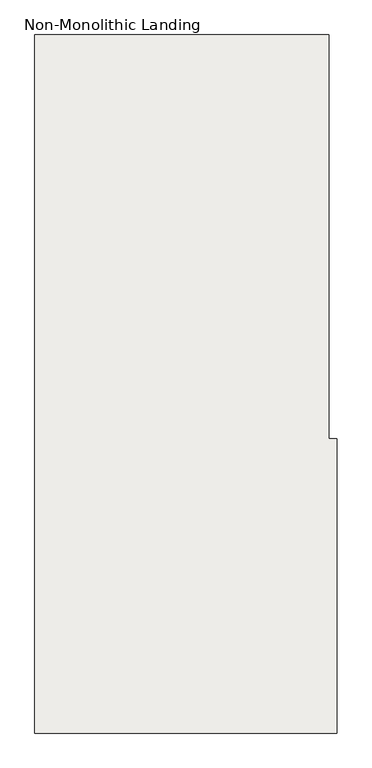
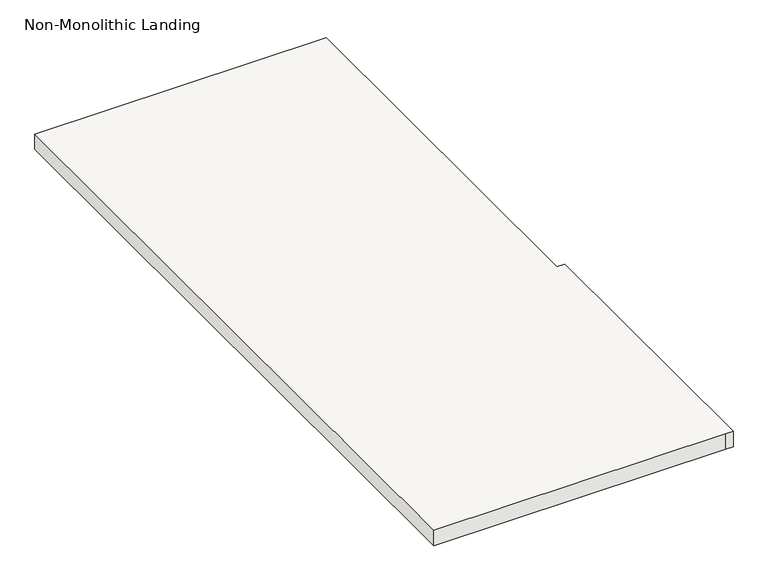
"""IFC4 building model written with IfcOpenShell, lengths in millimetres: slab geometry, Non-Monolithic Landing."""

from ifc_helpers import new_model, si_unit, origin, place, context, project, spatial, faceted_brep, source, transform, mapped, element, save


def non_monolithic_landing_bb243dde(model_context):
    return source(origin(), model_context, "Body", "Brep", [
        faceted_brep([(-12083.8120641, -2647.9669819, 8743.95), (-12058.4120641, -2647.9669819, 8769.35), (-12058.4120641, -3562.3669819, 8769.35), (-12083.8120641, -3562.3669819, 8743.95), (-12972.8120641, -2647.9669819, 8788.4), (-12972.8120641, -4817.9038196, 8788.4), (-12058.4120641, -4817.9038196, 8788.4), (-12033.0120641, -4817.9038196, 8788.4), (-12033.0120641, -3903.5038196, 8788.4), (-12058.4120641, -3903.5038196, 8788.4), (-12058.4120641, -2647.9669819, 8788.4), (-12083.8120641, -3562.3669819, 8737.6), (-12058.4120641, -3562.3669819, 8737.6), (-12058.4120641, -3903.5038196, 8737.6), (-12033.0120641, -3903.5038196, 8737.6), (-12033.0120641, -4817.9038196, 8737.6), (-12058.4120641, -4817.9038196, 8737.6), (-12972.8120641, -4817.9038196, 8737.6), (-12972.8120641, -2647.9669819, 8737.6), (-12083.8120641, -2647.9669819, 8737.6)], [[[0, 1, 2, 3]], [[4, 5, 6, 7, 8, 9, 10]], [[11, 12, 13, 14, 15, 16, 17, 18, 19]], [[12, 11, 3, 2]], [[11, 19, 0, 3]], [[4, 10, 1, 0, 19, 18]], [[5, 4, 18, 17]], [[6, 5, 17, 16]], [[7, 6, 16, 15]], [[8, 7, 15, 14]], [[9, 8, 14, 13]], [[10, 9, 13, 12, 2, 1]]]),
    ])


if __name__ == "__main__":
    model = new_model("IFC4")
    model_context = context("Model", 3, world=origin())
    ifc_project = project(units=[si_unit("LENGTHUNIT", "METRE", prefix="MILLI")], contexts=[model_context])
    site = spatial("IfcSite", under=ifc_project)
    building = spatial("IfcBuilding", under=site)
    placement = place(None, origin())
    non_monolithic_landing_shape = non_monolithic_landing_bb243dde(model_context)
    element("IfcSlab", 1, ObjectType="Non-Monolithic Landing", at=placement, inside=building, context=model_context, shape_type="MappedRepresentation", body=[
        mapped(non_monolithic_landing_shape, transform((0.0, 0.0, 0.0), x_axis=(1.0, 0.0, 0.0), y_axis=(0.0, 1.0, 0.0), z_axis=(0.0, 0.0, 1.0))),
    ])
    save(model, "model.ifc")
